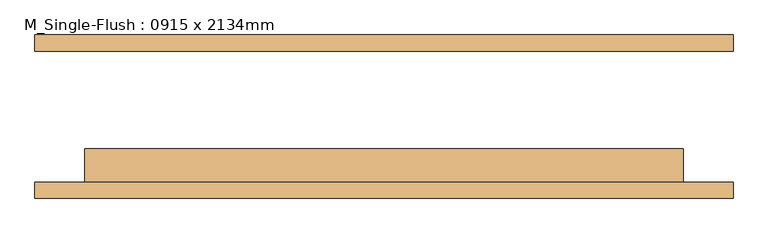
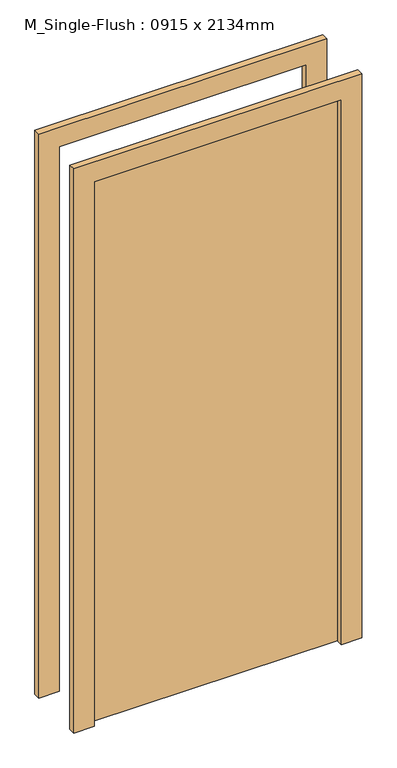
"""IFC4 building model written with IfcOpenShell, lengths in millimetres: door geometry, M_Single-Flush : 0915 x 2134mm."""

from ifc_helpers import new_model, si_unit, frame, origin, origin_with_axes, place, context, project, spatial, polyline, outline, extrude, source, transform, mapped, element, save


def m_single_flush_0915_x_2134mm_727434cd(model_context):
    return source(origin(), model_context, "Body", "SweptSolid", [
        extrude(outline(polyline([(2210.0, -533.5), (0.0, -533.5), (0.0, -457.5), (2134.0, -457.5), (2134.0, 457.5), (0.0, 457.5), (0.0, 533.5), (2210.0, 533.5), (2210.0, -533.5)])), frame((0.0, -125.0, 0.0), z_axis=(0.0, 1.0, 0.0), x_axis=(0.0, 0.0, 1.0)), (0.0, 0.0, 1.0), 25.0),
        extrude(outline(polyline([(2210.0, 533.5), (2210.0, -533.5), (0.0, -533.5), (0.0, -457.5), (2134.0, -457.5), (2134.0, 457.5), (0.0, 457.5), (0.0, 533.5), (2210.0, 533.5)])), frame((0.0, 100.0, 0.0), z_axis=(0.0, 1.0, 0.0), x_axis=(0.0, 0.0, 1.0)), (0.0, 0.0, 1.0), 25.0),
        extrude(outline(polyline([(457.5, -49.0), (457.5, -100.0), (-457.5, -100.0), (-457.5, -49.0), (457.5, -49.0)])), origin_with_axes(), (0.0, 0.0, 1.0), 2134.0),
    ])


if __name__ == "__main__":
    model = new_model("IFC4")
    model_context = context("Model", 3, world=origin())
    ifc_project = project(units=[si_unit("LENGTHUNIT", "METRE", prefix="MILLI")], contexts=[model_context])
    site = spatial("IfcSite", under=ifc_project)
    building = spatial("IfcBuilding", under=site)
    placement = place(None, origin())
    m_single_flush_0915_x_2134mm_shape = m_single_flush_0915_x_2134mm_727434cd(model_context)
    element("IfcDoor", 1, ObjectType="M_Single-Flush : 0915 x 2134mm", at=placement, inside=building, context=model_context, shape_type="MappedRepresentation", body=[
        mapped(m_single_flush_0915_x_2134mm_shape, transform((0.0, 0.0, 0.0), x_axis=(1.0, 0.0, 0.0), y_axis=(0.0, 1.0, 0.0), z_axis=(0.0, 0.0, 1.0))),
    ])
    save(model, "model.ifc")

# Revit data of these elements
# Type "M_Single-Flush : 0915 x 2134mm"
#   Type Mark = "15"
#   Thickness = 51 mm
#   Height = 2134 mm
#   Trim Projection Ext = 25 mm
#   Trim Projection Int = 25 mm
#   Trim Width = 76 mm
#   Width = 915 mm
#   Door Material = Door - Panel
#   Frame Material = Door - Frame
#   Function = (empty or 0)
#   Wall Closure = (empty or 0)
# Element 1 (IfcDoor, "M_Single-Flush : 0915 x 2134mm")
#   Materials on its faces: "Door - Frame", "Door - Panel"
# Materials
#   "Door - Panel": class "Wood", colour RGB 114 82 51, transparency 0
#   "Door - Frame": colour RGB 153 76 43, transparency 0
